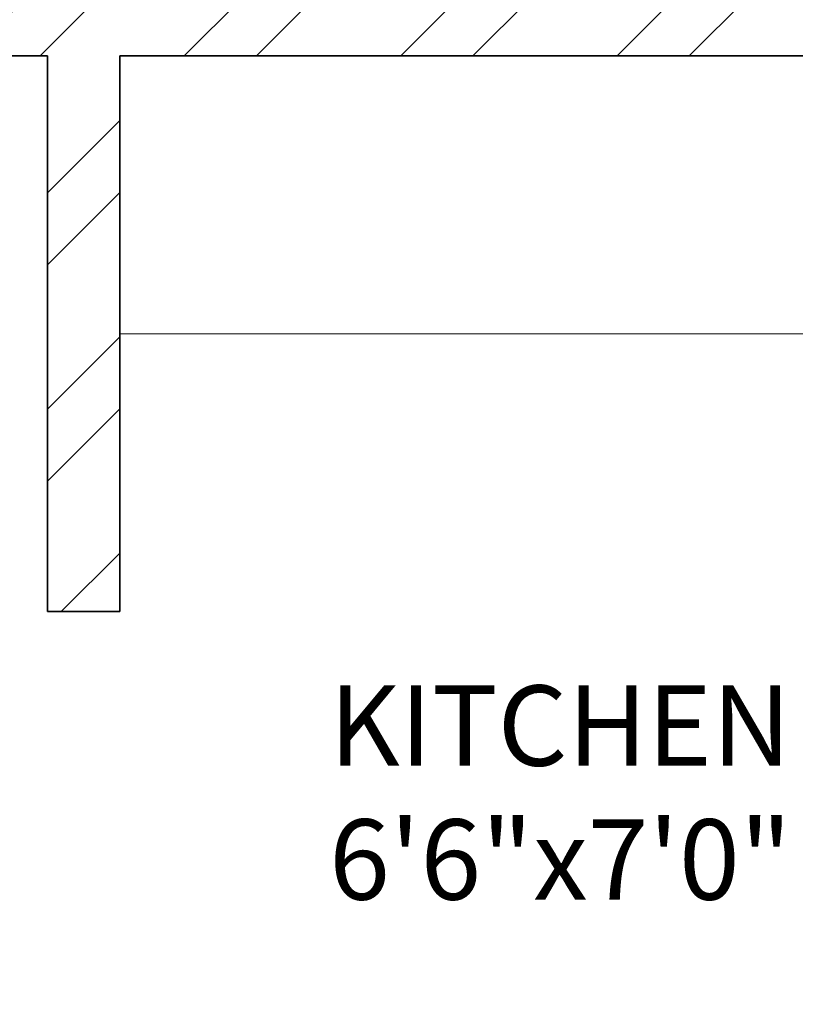
# Model space of a CAD drawing. Units: inches. Extents: x 2168 to 3056, y 1130 to 2629.
# Tile 17 of 42: x 2780 to 2828, y 2017 to 2079. Entities that reach past the tile are written whole.
import ezdxf

# ---------------------------------------------------------------- set-up
doc = ezdxf.new("R2010")
doc.units = ezdxf.units.IN
for name, color, linetype, lineweight in [('A-AREA-IDEN', 7, 'Continuous', 18), ('A-FLOR-CASE', 71, 'Continuous', 18), ('A-WALL', 7, 'Continuous', 35)]:
    doc.layers.add(name, color=color, linetype=linetype, lineweight=lineweight)
doc.layers.add('A-WALL-PATT', color=143, linetype='Continuous', lineweight=13, true_color=0x7aafdf)
doc.styles.get("Standard").update_dxf_attribs({"font": 'arial.ttf'})

msp = doc.modelspace()

# ---------------------------------------------------------------- hatches: boundary and pattern name
at = {"layer": 'A-WALL-PATT'}
h = msp.add_hatch(dxfattribs=at)
h.set_pattern_fill('ANSI32', color=256)
h.paths.add_polyline_path([(2463.796, 2409.389), (2467.387, 2409.389), (2467.387, 2413.889), (2454.768, 2413.889), (2454.768, 2411.639), (2454.768, 2409.389), (2459.296, 2409.389), (2459.296, 2265.389), (2455.644, 2265.389), (2455.644, 2260.889), (2467.349, 2260.889), (2467.349, 2263.139), (2467.349, 2265.389), (2463.796, 2265.389)])
h.paths.add_polyline_path([(2431.596, 2413.889), (2409.647, 2413.889), (2409.647, 2409.389), (2431.596, 2409.389), (2431.596, 2411.639)])
h.paths.add_polyline_path([(2349.647, 2413.889), (2331.796, 2413.889), (2331.796, 2362.671), (2336.296, 2362.671), (2336.296, 2409.389), (2349.647, 2409.389), (2349.647, 2411.639)])
h.paths.add_polyline_path([(2634.149, 2411.639), (2634.149, 2413.889), (2562.293, 2413.889), (2562.293, 2409.389), (2595.796, 2409.389), (2595.796, 2280.309), (2595.826, 2280.309), (2595.826, 2265.389), (2499.91, 2265.389), (2499.91, 2260.889), (2550.796, 2260.889), (2550.796, 2117.308), (2555.296, 2117.308), (2555.296, 2168.08), (2571.93, 2168.08), (2571.93, 2176.889), (2559.796, 2176.889), (2559.796, 2256.389), (2640.796, 2256.389), (2640.796, 2176.889), (2626.428, 2176.889), (2626.428, 2168.08), (2645.296, 2168.08), (2645.296, 2116.637), (2649.796, 2116.637), (2649.796, 2260.889), (2691.251, 2260.889), (2691.251, 2263.139), (2691.251, 2265.389), (2670.655, 2265.389), (2670.655, 2265.365), (2600.296, 2265.365), (2600.296, 2280.258), (2600.296, 2409.389), (2634.149, 2409.389)])
h.paths.add_polyline_path([(2600.296, 2473.889), (2612.84, 2473.889), (2612.84, 2478.389), (2572.636, 2478.389), (2572.636, 2473.889), (2595.796, 2473.889), (2595.796, 2413.889), (2600.296, 2413.889)])
h.paths.add_polyline_path([(2535.796, 2473.889), (2548.636, 2473.889), (2548.636, 2478.389), (2531.396, 2478.389), (2531.396, 2413.889), (2521.6, 2413.889), (2521.6, 2409.389), (2539.239, 2409.389), (2539.239, 2411.639), (2539.239, 2413.889), (2535.796, 2413.889)])
h.paths.add_polyline_path([(2664.796, 2478.389), (2636.84, 2478.389), (2636.84, 2473.889), (2660.296, 2473.889), (2660.296, 2413.889), (2656.165, 2413.889), (2656.165, 2409.389), (2671.684, 2409.389), (2671.684, 2411.639), (2671.684, 2413.889), (2664.796, 2413.889)])
h.paths.add_polyline_path([(2705.942, 2413.889), (2695.684, 2413.889), (2695.684, 2409.389), (2705.942, 2409.389)])
h.paths.add_polyline_path([(2741.35, 2413.889), (2728.733, 2413.889), (2728.733, 2411.639), (2728.733, 2409.389), (2732.296, 2409.389), (2732.296, 2265.389), (2725.733, 2265.389), (2725.733, 2260.889), (2740.917, 2260.889), (2740.917, 2263.139), (2740.917, 2265.389), (2736.796, 2265.389), (2736.796, 2409.389), (2741.35, 2409.389)])
h.paths.add_polyline_path([(2785.655, 2413.889), (2764.546, 2413.889), (2764.486, 2409.389), (2785.655, 2409.389), (2785.655, 2411.639)])
h.paths.add_polyline_path([(2864.296, 2413.889), (2845.655, 2413.889), (2845.655, 2409.389), (2859.796, 2409.389), (2859.796, 2368.425), (2864.296, 2368.425)])
h.paths.add_polyline_path([(2864.296, 2308.425), (2862.046, 2308.425), (2859.796, 2308.425), (2859.796, 2265.389), (2774.483, 2265.389), (2774.483, 2263.139), (2774.483, 2260.889), (2781.796, 2260.889), (2781.796, 2226.654), (2786.296, 2226.654), (2786.296, 2260.889), (2859.796, 2260.889), (2859.796, 2241.352), (2864.296, 2241.352)])
h.paths.add_polyline_path([(2864.296, 2217.352), (2862.046, 2217.352), (2859.796, 2217.352), (2859.796, 2200.889), (2786.296, 2200.889), (2786.296, 2205.931), (2784.046, 2205.931), (2781.796, 2205.931), (2781.796, 2150.974), (2786.296, 2150.974), (2786.296, 2161.889), (2859.796, 2161.889), (2859.796, 2144.419), (2864.296, 2144.419)])
h.paths.add_polyline_path([(2859.796, 2196.389), (2859.796, 2166.389), (2786.296, 2166.389), (2786.296, 2196.389)], flags=16)
h.paths.add_polyline_path([(2864.296, 2108.419), (2862.046, 2108.419), (2859.796, 2108.419), (2859.796, 2080.889), (2786.296, 2080.889), (2786.296, 2111.993), (2781.796, 2111.993), (2781.796, 2080.889), (2649.796, 2080.889), (2649.796, 2086.036), (2647.546, 2086.036), (2645.296, 2086.036), (2645.296, 2071.739), (2649.796, 2071.739), (2649.796, 2076.389), (2781.796, 2076.389), (2781.796, 2041.792), (2786.296, 2041.792), (2786.296, 2076.389), (2859.796, 2076.389), (2859.796, 2058.577), (2864.296, 2058.577)])
h.paths.add_polyline_path([(2864.296, 2022.577), (2859.796, 2022.577), (2859.796, 1992.389), (2786.296, 1992.389), (2786.296, 1999.573), (2781.796, 1999.573), (2781.796, 1848.085), (2784.046, 1848.085), (2786.296, 1848.085), (2786.296, 1851.389), (2859.796, 1851.389), (2859.796, 1838.258), (2864.296, 1838.258)], flags=17)
h.paths.add_polyline_path([(2859.796, 1987.889), (2859.796, 1855.889), (2786.296, 1855.889), (2786.296, 1987.889)], flags=16)
h.paths.add_polyline_path([(2823.046, 1987.889), (2841.421, 1921.889), (2823.046, 1855.889)], flags=0)
h.paths.add_polyline_path([(2864.296, 1814.258), (2859.796, 1814.258), (2859.796, 1791.389), (2786.296, 1791.389), (2786.296, 1825.658), (2784.046, 1825.658), (2781.796, 1825.658), (2781.796, 1791.389), (2720.155, 1791.389), (2720.155, 1791.265), (2649.796, 1791.265), (2649.796, 1806.159), (2649.796, 2038.983), (2647.546, 2038.983), (2645.296, 2038.983), (2645.296, 1783.925), (2649.796, 1783.925), (2649.796, 1786.889), (2781.796, 1786.889), (2781.796, 1746.789), (2786.296, 1746.789), (2786.296, 1786.889), (2859.796, 1786.889), (2859.796, 1770.083), (2864.296, 1770.083)])
h.paths.add_polyline_path([(2864.296, 1734.083), (2862.046, 1734.083), (2859.796, 1734.083), (2859.796, 1705.889), (2786.296, 1705.889), (2786.296, 1714.166), (2781.796, 1714.166), (2781.796, 1660.527), (2786.296, 1660.527), (2786.296, 1666.889), (2859.796, 1666.889), (2859.796, 1648.342), (2864.296, 1648.342)])
h.paths.add_polyline_path([(2786.296, 1701.389), (2859.796, 1701.389), (2859.796, 1671.389), (2786.296, 1671.389)], flags=16)
h.paths.add_polyline_path([(2649.796, 1756.576), (2647.546, 1756.576), (2645.296, 1756.576), (2645.296, 1606.889), (2555.296, 1606.889), (2555.296, 1749.513), (2553.046, 1749.513), (2550.796, 1749.513), (2550.796, 1606.889), (2503.006, 1606.889), (2503.006, 1604.639), (2503.006, 1602.389), (2595.796, 1602.389), (2595.849, 1602.389), (2595.849, 1587.495), (2595.796, 1458.389), (2561.502, 1458.389), (2561.502, 1456.139), (2561.502, 1453.889), (2595.796, 1453.889), (2595.796, 1381.889), (2573.438, 1381.889), (2573.438, 1377.389), (2613.01, 1377.389), (2613.01, 1379.639), (2613.01, 1381.889), (2600.296, 1381.889), (2600.296, 1453.889), (2634.327, 1453.889), (2634.327, 1458.389), (2600.296, 1458.389), (2600.296, 1602.389), (2670.655, 1602.389), (2694.095, 1602.389), (2694.095, 1606.889), (2649.796, 1606.889)])
h.paths.add_polyline_path([(2736.796, 1602.389), (2741.562, 1602.389), (2741.562, 1606.889), (2726.203, 1606.889), (2726.203, 1604.639), (2726.203, 1602.389), (2732.296, 1602.389), (2732.296, 1458.389), (2727.899, 1458.389), (2727.899, 1453.889), (2740.821, 1453.889), (2740.821, 1456.139), (2740.821, 1458.389), (2736.796, 1458.389)])
h.paths.add_polyline_path([(2859.796, 1606.889), (2786.296, 1606.889), (2786.296, 1637.334), (2784.046, 1637.334), (2781.796, 1637.334), (2781.796, 1606.889), (2775.612, 1606.889), (2775.612, 1602.389), (2859.796, 1602.389)])
h.paths.add_polyline_path([(2864.296, 1624.342), (2862.046, 1624.342), (2859.796, 1624.342), (2859.796, 1570.39), (2864.296, 1570.39)])
h.paths.add_polyline_path([(2864.296, 1510.39), (2862.046, 1510.39), (2859.796, 1510.39), (2859.796, 1458.389), (2846.735, 1458.389), (2846.735, 1456.139), (2846.735, 1453.889), (2864.296, 1453.889)])
h.paths.add_polyline_path([(2786.735, 1458.389), (2765.444, 1458.389), (2765.444, 1453.889), (2786.735, 1453.889)])
h.paths.add_polyline_path([(2706.004, 1458.389), (2695.36, 1458.389), (2695.36, 1453.889), (2706.004, 1453.889), (2706.004, 1456.139)])
h.paths.add_polyline_path([(2671.36, 1456.139), (2671.36, 1458.389), (2655.986, 1458.389), (2655.986, 1456.139), (2655.986, 1453.889), (2660.296, 1453.889), (2660.296, 1381.889), (2637.01, 1381.889), (2637.01, 1377.389), (2664.796, 1377.389), (2664.796, 1453.889), (2671.36, 1453.889)], flags=17)
h.paths.add_polyline_path([(2539.829, 1458.389), (2520.237, 1458.389), (2520.237, 1453.889), (2531.296, 1453.889), (2531.296, 1377.389), (2546.449, 1377.389), (2546.449, 1379.639), (2546.449, 1381.889), (2535.796, 1381.889), (2535.796, 1453.889), (2539.829, 1453.889)], flags=17)
h.paths.add_polyline_path([(2496.237, 1458.389), (2489.13, 1458.389), (2489.13, 1453.889), (2496.237, 1453.889), (2496.237, 1456.139)])
h.paths.add_polyline_path([(2467.433, 1456.139), (2467.433, 1458.389), (2463.796, 1458.389), (2463.796, 1602.389), (2468.242, 1602.389), (2468.242, 1605.7), (2468.242, 1606.889), (2454.602, 1606.889), (2454.602, 1602.389), (2459.296, 1602.389), (2459.296, 1458.389), (2454.24, 1458.389), (2454.24, 1453.889), (2467.433, 1453.889)])
h.paths.add_polyline_path([(2431.601, 1456.139), (2431.601, 1458.389), (2411.386, 1458.389), (2411.386, 1453.889), (2431.601, 1453.889)])
h.paths.add_polyline_path([(2351.386, 1458.389), (2336.296, 1458.389), (2336.296, 1490.693), (2334.046, 1490.693), (2331.796, 1490.693), (2331.796, 1453.889), (2351.386, 1453.889), (2351.386, 1456.139)])
h.paths.add_polyline_path([(2336.296, 1629.705), (2331.796, 1629.705), (2331.796, 1552.317), (2336.296, 1552.317), (2336.296, 1602.389), (2406.655, 1602.389), (2423.472, 1602.389), (2423.472, 1606.889), (2418.796, 1606.889), (2418.796, 1643.678), (2416.546, 1643.678), (2414.296, 1643.678), (2414.296, 1606.889), (2336.296, 1606.889)])
h.paths.add_polyline_path([(2418.796, 1714.384), (2414.296, 1714.384), (2414.296, 1705.889), (2336.296, 1705.889), (2336.296, 1731.324), (2334.046, 1731.324), (2331.796, 1731.324), (2331.796, 1653.705), (2334.046, 1653.705), (2336.296, 1653.705), (2336.296, 1666.889), (2414.296, 1666.889), (2414.296, 1663.589), (2418.796, 1663.589)])
h.paths.add_polyline_path([(2336.296, 1701.389), (2414.296, 1701.389), (2414.296, 1671.389), (2336.296, 1671.389)], flags=16)
h.paths.add_polyline_path([(2555.296, 2040.059), (2550.796, 2040.059), (2550.796, 1791.389), (2550.561, 1791.205), (2480.202, 1791.205), (2418.796, 1791.389), (2418.796, 1825.448), (2416.546, 1825.448), (2414.296, 1825.448), (2414.296, 1791.389), (2336.296, 1791.389), (2336.296, 1806.409), (2331.796, 1806.409), (2331.796, 1767.324), (2336.296, 1767.324), (2336.296, 1786.889), (2414.296, 1786.889), (2414.296, 1745.457), (2418.796, 1745.457), (2418.796, 1786.889), (2550.796, 1786.889), (2550.796, 1783.011), (2555.296, 1783.011)])
h.paths.add_polyline_path([(2418.796, 1923.389), (2423.207, 1923.389), (2423.207, 1925.639), (2423.207, 1927.889), (2418.796, 1927.889), (2418.796, 2000.048), (2414.296, 2000.048), (2414.296, 1992.389), (2336.296, 1992.389), (2336.296, 1987.889), (2414.296, 1987.889), (2414.296, 1855.889), (2336.296, 1855.889), (2336.296, 1851.389), (2414.296, 1851.389), (2414.296, 1846.759), (2418.796, 1846.759)], flags=17)
h.paths.add_polyline_path([(2336.296, 2019.294), (2334.046, 2019.294), (2331.796, 2019.294), (2331.796, 1830.409), (2336.296, 1830.409)], flags=17)
h.paths.add_polyline_path([(2550.796, 1927.889), (2453.541, 1927.889), (2453.541, 1925.639), (2453.541, 1923.389), (2550.796, 1923.389)], flags=17)
h.paths.add_polyline_path([(2744.987, 1927.889), (2649.796, 1927.889), (2649.796, 1923.389), (2744.987, 1923.389), (2744.987, 1925.639)], flags=17)
h.paths.add_polyline_path([(2555.296, 2086.458), (2553.046, 2086.458), (2550.796, 2086.458), (2550.796, 2080.889), (2418.796, 2080.889), (2336.296, 2080.889), (2336.296, 2115.399), (2334.046, 2115.399), (2331.796, 2115.399), (2331.796, 2055.294), (2336.296, 2055.294), (2336.296, 2076.389), (2550.796, 2076.389), (2550.796, 2071.538), (2555.296, 2071.538)])
h.paths.add_polyline_path([(2418.796, 2121.389), (2414.296, 2121.389), (2414.296, 2080.889), (2418.796, 2080.889)])
h.paths.add_polyline_path([(2418.796, 2076.389), (2414.296, 2076.389), (2414.296, 2035.123), (2418.796, 2035.123)])
h.paths.add_polyline_path([(2422.868, 2263.139), (2422.868, 2265.389), (2406.655, 2265.389), (2406.655, 2265.359), (2336.296, 2265.359), (2336.296, 2280.252), (2336.296, 2302.671), (2334.046, 2302.671), (2331.796, 2302.671), (2331.796, 2246.853), (2336.296, 2246.853), (2336.296, 2260.889), (2414.296, 2260.889), (2414.296, 2223.996), (2418.796, 2223.996), (2418.796, 2260.889), (2422.868, 2260.889)])
h.paths.add_polyline_path([(2418.796, 2204.783), (2416.546, 2204.783), (2414.296, 2204.783), (2414.296, 2200.889), (2336.296, 2200.889), (2336.296, 2220.853), (2331.796, 2220.853), (2331.796, 2151.399), (2336.296, 2151.399), (2336.296, 2161.889), (2414.296, 2161.889), (2414.296, 2153.726), (2418.796, 2153.726)])
h.paths.add_polyline_path([(2414.296, 2196.389), (2414.296, 2166.389), (2336.296, 2166.389), (2336.296, 2196.389)], flags=16)
h.paths.add_polyline_path([(2375.296, 2181.389), (2336.296, 2166.389), (2336.296, 2196.389)], flags=0)
h.paths.add_polyline_path([(2809.595, 2172.34), (2838.804, 2172.34), (2838.804, 2190.997), (2809.595, 2190.997)], flags=8)
h.paths.add_polyline_path([(2849.75, 1919.585), (2849.75, 1952.672), (2831.093, 1952.672), (2831.093, 1919.585)], flags=8)
h.paths.add_polyline_path([(2808.875, 1901.967), (2808.875, 1937.85), (2790.149, 1937.85), (2790.149, 1901.967)], flags=8)
h.paths.add_polyline_path([(2806.285, 1671.896), (2835.493, 1671.896), (2835.493, 1690.553), (2806.285, 1690.553)], flags=8)
h.paths.add_polyline_path([(2353.186, 1676.549), (2382.395, 1676.549), (2382.395, 1695.207), (2353.186, 1695.207)], flags=8)
h.paths.add_polyline_path([(2360.083, 1832.308), (2389.241, 1832.308), (2389.241, 1850.966), (2360.083, 1850.966)], flags=25)
h.paths.add_polyline_path([(2354.822, 2167.823), (2384.031, 2167.823), (2384.031, 2186.481), (2354.822, 2186.481)], flags=8)

# ---------------------------------------------------------------- linework, layer by layer
at = {"layer": 'A-FLOR-CASE'}
msp.add_line((2786.296, 2059.09), (2844.993, 2059.09), dxfattribs=at)
at = {"layer": 'A-WALL'}
for p, q in [((2649.796, 2076.389), (2781.796, 2076.389)), ((2781.796, 2076.389), (2781.796, 2041.792)), ((2786.296, 2076.389), (2786.296, 2041.792)), ((2786.296, 2076.389), (2859.796, 2076.389)), ((2781.796, 2041.792), (2786.296, 2041.792))]:
    msp.add_line(p, q, dxfattribs=at)

# ---------------------------------------------------------------- texts
at = {"layer": 'A-AREA-IDEN', "insert": (2799.333, 2037.189), "char_height": 5, "attachment_point": 1}
msp.add_mtext_dynamic_manual_height_columns('KITCHEN\\P6\'6"x7\'0"', width=128.86731, gutter_width=12.5, heights=[0], dxfattribs=at)

doc.saveas('drawing.dxf')
